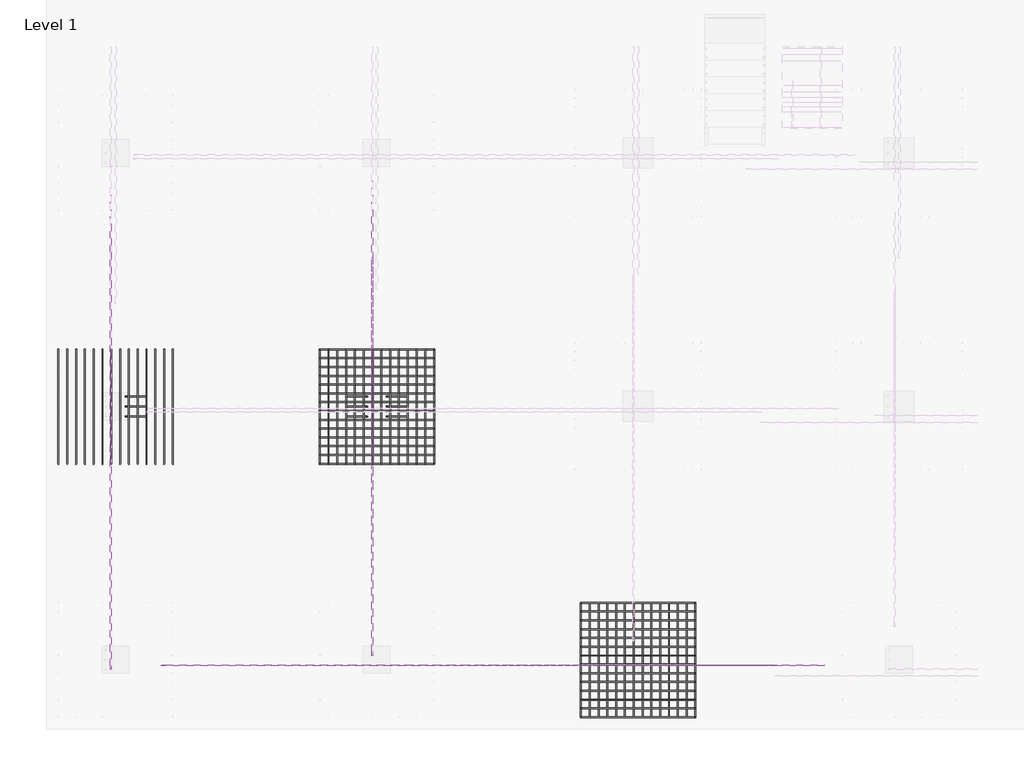
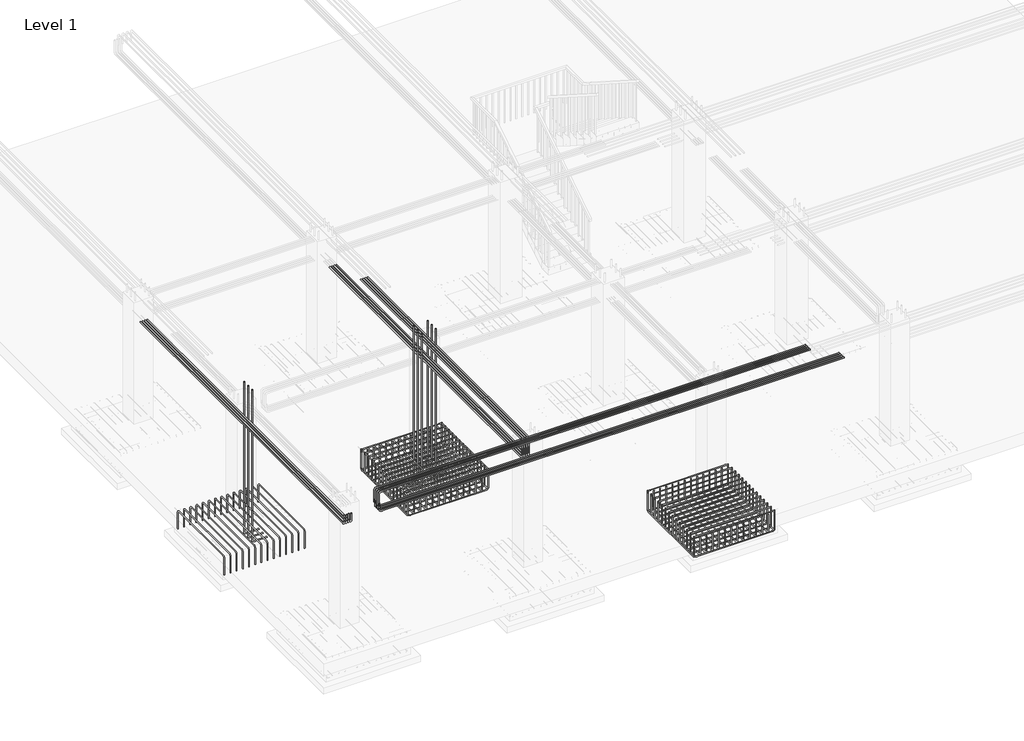
# One storey, part 4 of 17: 21 reinforcing bars.
"""IFC4 building model written with IfcOpenShell, lengths in millimetres."""

from ifc_helpers import new_model, si_unit, point, frame, origin, place, context, project, spatial, polyline, circle_curve, trimmed, segment, composite_curve, source, transform, mapped, element, save
from ifc_brep_helpers import swept_disk

model = new_model("IFC4")

# Units and contexts
model_context = context("Model", 3, world=origin())
ifc_project = project(units=[si_unit("LENGTHUNIT", "METRE", prefix="MILLI")], contexts=[model_context])

# Site, building, storey
site = spatial("IfcSite", under=ifc_project)
building = spatial("IfcBuilding", under=site)
storey = spatial("IfcBuildingStorey", under=building, Name="Level 1", Elevation=0.0)

# Reinforcing bars
placement = place(None, origin())
reinforcing_bar_shape = source(origin(), model_context, "Body", "SolidModel", [
    swept_disk(composite_curve([segment(polyline([(-13686.3632003, 636.009457, -504.0), (-13686.3632003, 636.009457, -96.0)]), True, "CONTINUOUS"), segment(trimmed(circle_curve(frame((-13686.3632003, 588.009457, -96.0), z_axis=(1.0, 0.0, 0.0), x_axis=(0.0, 48.0, 0.0)), 48.0), [point((-13686.3632003, 636.009457, -96.0))], [point((-13686.3632003, 588.009457, -48.0))], True, "CARTESIAN"), True, "CONTINUOUS"), segment(polyline([(-13686.3632003, 588.009457, -48.0), (-13686.3632003, -1219.990543, -48.0)]), True, "CONTINUOUS"), segment(trimmed(circle_curve(frame((-13686.3632003, -1219.990543, -96.0), z_axis=(1.0, 0.0, 0.0), x_axis=(0.0, 0.0, 48.0)), 48.0), [point((-13686.3632003, -1219.990543, -48.0))], [point((-13686.3632003, -1267.990543, -96.0))], True, "CARTESIAN"), True, "CONTINUOUS"), segment(polyline([(-13686.3632003, -1267.990543, -96.0), (-13686.3632003, -1267.990543, -504.0)]), True, "CONTINUOUS")], self_intersect=False), 8.0),
])
element("IfcReinforcingBar", 1, at=placement, inside=storey, context=model_context, shape_type="MappedRepresentation", body=[
    mapped(reinforcing_bar_shape, transform((0.0, 0.0, 0.0), x_axis=(1.0, 0.0, 0.0), y_axis=(0.0, 1.0, 0.0), z_axis=(0.0, 0.0, 1.0))),
    mapped(reinforcing_bar_shape, transform((146.4615385, 0.0, 0.0), x_axis=(1.0, 0.0, 0.0), y_axis=(0.0, 1.0, 0.0), z_axis=(0.0, 0.0, 1.0))),
    mapped(reinforcing_bar_shape, transform((292.9230769, 0.0, 0.0), x_axis=(1.0, 0.0, 0.0), y_axis=(0.0, 1.0, 0.0), z_axis=(0.0, 0.0, 1.0))),
    mapped(reinforcing_bar_shape, transform((439.3846154, 0.0, 0.0), x_axis=(1.0, 0.0, 0.0), y_axis=(0.0, 1.0, 0.0), z_axis=(0.0, 0.0, 1.0))),
    mapped(reinforcing_bar_shape, transform((585.8461538, 0.0, 0.0), x_axis=(1.0, 0.0, 0.0), y_axis=(0.0, 1.0, 0.0), z_axis=(0.0, 0.0, 1.0))),
    mapped(reinforcing_bar_shape, transform((732.3076923, 0.0, 0.0), x_axis=(1.0, 0.0, 0.0), y_axis=(0.0, 1.0, 0.0), z_axis=(0.0, 0.0, 1.0))),
    mapped(reinforcing_bar_shape, transform((878.7692308, 0.0, 0.0), x_axis=(1.0, 0.0, 0.0), y_axis=(0.0, 1.0, 0.0), z_axis=(0.0, 0.0, 1.0))),
    mapped(reinforcing_bar_shape, transform((1025.2307692, 0.0, 0.0), x_axis=(1.0, 0.0, 0.0), y_axis=(0.0, 1.0, 0.0), z_axis=(0.0, 0.0, 1.0))),
    mapped(reinforcing_bar_shape, transform((1171.6923077, 0.0, 0.0), x_axis=(1.0, 0.0, 0.0), y_axis=(0.0, 1.0, 0.0), z_axis=(0.0, 0.0, 1.0))),
    mapped(reinforcing_bar_shape, transform((1318.1538462, 0.0, 0.0), x_axis=(1.0, 0.0, 0.0), y_axis=(0.0, 1.0, 0.0), z_axis=(0.0, 0.0, 1.0))),
    mapped(reinforcing_bar_shape, transform((1464.6153846, 0.0, 0.0), x_axis=(1.0, 0.0, 0.0), y_axis=(0.0, 1.0, 0.0), z_axis=(0.0, 0.0, 1.0))),
    mapped(reinforcing_bar_shape, transform((1611.0769231, 0.0, 0.0), x_axis=(1.0, 0.0, 0.0), y_axis=(0.0, 1.0, 0.0), z_axis=(0.0, 0.0, 1.0))),
    mapped(reinforcing_bar_shape, transform((1757.5384615, 0.0, 0.0), x_axis=(1.0, 0.0, 0.0), y_axis=(0.0, 1.0, 0.0), z_axis=(0.0, 0.0, 1.0))),
    mapped(reinforcing_bar_shape, transform((1904.0, 0.0, 0.0), x_axis=(1.0, 0.0, 0.0), y_axis=(0.0, 1.0, 0.0), z_axis=(0.0, 0.0, 1.0))),
])
reinforcing_bar_2_shape = source(origin(), model_context, "Body", "SolidModel", [
    swept_disk(composite_curve([segment(polyline([(-12221.7478157, -481.490543, -550.0), (-12518.8632003, -481.490543, -550.0)]), True, "CONTINUOUS"), segment(trimmed(circle_curve(frame((-12518.8632003, -481.490543, -500.0), z_axis=(0.0, 1.0, 0.0), x_axis=(0.0, 0.0, -50.0)), 50.0), [point((-12518.8632003, -481.490543, -550.0))], [point((-12568.8632003, -481.490543, -500.0))], True, "CARTESIAN"), True, "CONTINUOUS"), segment(polyline([(-12568.8632003, -481.490543, -500.0), (-12568.8632003, -481.490543, 3260.0)]), True, "CONTINUOUS")], self_intersect=False), 10.0),
])
element("IfcReinforcingBar", 2, at=placement, inside=storey, context=model_context, shape_type="MappedRepresentation", body=[
    mapped(reinforcing_bar_2_shape, transform((0.0, 0.0, 0.0), x_axis=(1.0, 0.0, 0.0), y_axis=(0.0, 1.0, 0.0), z_axis=(0.0, 0.0, 1.0))),
    mapped(reinforcing_bar_2_shape, transform((0.0, 165.5, 0.0), x_axis=(1.0, 0.0, 0.0), y_axis=(0.0, 1.0, 0.0), z_axis=(0.0, 0.0, 1.0))),
    mapped(reinforcing_bar_2_shape, transform((0.0, 331.0, 0.0), x_axis=(1.0, 0.0, 0.0), y_axis=(0.0, 1.0, 0.0), z_axis=(0.0, 0.0, 1.0))),
])
reinforcing_bar_3_shape = source(origin(), model_context, "Body", "SolidModel", [
    swept_disk(composite_curve([segment(polyline([(-9341.3632003, 636.009457, -40.0), (-9341.3632003, 636.009457, -504.0)]), True, "CONTINUOUS"), segment(trimmed(circle_curve(frame((-9293.3632003, 636.009457, -504.0), z_axis=(0.0, -1.0, 0.0), x_axis=(-48.0, 0.0, 0.0)), 48.0), [point((-9341.3632003, 636.009457, -504.0))], [point((-9293.3632003, 636.009457, -552.0))], True, "CARTESIAN"), True, "CONTINUOUS"), segment(polyline([(-9293.3632003, 636.009457, -552.0), (-7485.3632003, 636.009457, -552.0)]), True, "CONTINUOUS"), segment(trimmed(circle_curve(frame((-7485.3632003, 636.009457, -504.0), z_axis=(0.0, -1.0, 0.0), x_axis=(0.0, 0.0, -48.0)), 48.0), [point((-7485.3632003, 636.009457, -552.0))], [point((-7437.3632003, 636.009457, -504.0))], True, "CARTESIAN"), True, "CONTINUOUS"), segment(polyline([(-7437.3632003, 636.009457, -504.0), (-7437.3632003, 636.009457, -40.0)]), True, "CONTINUOUS")], self_intersect=False), 8.0),
])
element("IfcReinforcingBar", 3, at=placement, inside=storey, context=model_context, shape_type="MappedRepresentation", body=[
    mapped(reinforcing_bar_3_shape, transform((0.0, 0.0, 0.0), x_axis=(1.0, 0.0, 0.0), y_axis=(0.0, 1.0, 0.0), z_axis=(0.0, 0.0, 1.0))),
    mapped(reinforcing_bar_3_shape, transform((0.0, -146.4615385, 0.0), x_axis=(1.0, 0.0, 0.0), y_axis=(0.0, 1.0, 0.0), z_axis=(0.0, 0.0, 1.0))),
    mapped(reinforcing_bar_3_shape, transform((0.0, -292.9230769, 0.0), x_axis=(1.0, 0.0, 0.0), y_axis=(0.0, 1.0, 0.0), z_axis=(0.0, 0.0, 1.0))),
    mapped(reinforcing_bar_3_shape, transform((0.0, -439.3846154, 0.0), x_axis=(1.0, 0.0, 0.0), y_axis=(0.0, 1.0, 0.0), z_axis=(0.0, 0.0, 1.0))),
    mapped(reinforcing_bar_3_shape, transform((0.0, -585.8461538, 0.0), x_axis=(1.0, 0.0, 0.0), y_axis=(0.0, 1.0, 0.0), z_axis=(0.0, 0.0, 1.0))),
    mapped(reinforcing_bar_3_shape, transform((0.0, -732.3076923, 0.0), x_axis=(1.0, 0.0, 0.0), y_axis=(0.0, 1.0, 0.0), z_axis=(0.0, 0.0, 1.0))),
    mapped(reinforcing_bar_3_shape, transform((0.0, -878.7692308, 0.0), x_axis=(1.0, 0.0, 0.0), y_axis=(0.0, 1.0, 0.0), z_axis=(0.0, 0.0, 1.0))),
    mapped(reinforcing_bar_3_shape, transform((0.0, -1025.2307692, 0.0), x_axis=(1.0, 0.0, 0.0), y_axis=(0.0, 1.0, 0.0), z_axis=(0.0, 0.0, 1.0))),
    mapped(reinforcing_bar_3_shape, transform((0.0, -1171.6923077, 0.0), x_axis=(1.0, 0.0, 0.0), y_axis=(0.0, 1.0, 0.0), z_axis=(0.0, 0.0, 1.0))),
    mapped(reinforcing_bar_3_shape, transform((0.0, -1318.1538462, 0.0), x_axis=(1.0, 0.0, 0.0), y_axis=(0.0, 1.0, 0.0), z_axis=(0.0, 0.0, 1.0))),
    mapped(reinforcing_bar_3_shape, transform((0.0, -1464.6153846, 0.0), x_axis=(1.0, 0.0, 0.0), y_axis=(0.0, 1.0, 0.0), z_axis=(0.0, 0.0, 1.0))),
    mapped(reinforcing_bar_3_shape, transform((0.0, -1611.0769231, 0.0), x_axis=(1.0, 0.0, 0.0), y_axis=(0.0, 1.0, 0.0), z_axis=(0.0, 0.0, 1.0))),
    mapped(reinforcing_bar_3_shape, transform((0.0, -1757.5384615, 0.0), x_axis=(1.0, 0.0, 0.0), y_axis=(0.0, 1.0, 0.0), z_axis=(0.0, 0.0, 1.0))),
    mapped(reinforcing_bar_3_shape, transform((0.0, -1904.0, 0.0), x_axis=(1.0, 0.0, 0.0), y_axis=(0.0, 1.0, 0.0), z_axis=(0.0, 0.0, 1.0))),
])
reinforcing_bar_4_shape = source(origin(), model_context, "Body", "SolidModel", [
    swept_disk(composite_curve([segment(polyline([(-9341.3632003, -1267.990543, -504.0), (-9341.3632003, -1267.990543, -96.0)]), True, "CONTINUOUS"), segment(trimmed(circle_curve(frame((-9293.3632003, -1267.990543, -96.0), z_axis=(0.0, 1.0, 0.0), x_axis=(-48.0, 0.0, 0.0)), 48.0), [point((-9341.3632003, -1267.990543, -96.0))], [point((-9293.3632003, -1267.990543, -48.0))], True, "CARTESIAN"), True, "CONTINUOUS"), segment(polyline([(-9293.3632003, -1267.990543, -48.0), (-7485.3632003, -1267.990543, -48.0)]), True, "CONTINUOUS"), segment(trimmed(circle_curve(frame((-7485.3632003, -1267.990543, -96.0), z_axis=(0.0, 1.0, 0.0), x_axis=(0.0, 0.0, 48.0)), 48.0), [point((-7485.3632003, -1267.990543, -48.0))], [point((-7437.3632003, -1267.990543, -96.0))], True, "CARTESIAN"), True, "CONTINUOUS"), segment(polyline([(-7437.3632003, -1267.990543, -96.0), (-7437.3632003, -1267.990543, -504.0)]), True, "CONTINUOUS")], self_intersect=False), 8.0),
])
element("IfcReinforcingBar", 4, at=placement, inside=storey, context=model_context, shape_type="MappedRepresentation", body=[
    mapped(reinforcing_bar_4_shape, transform((0.0, 0.0, 0.0), x_axis=(1.0, 0.0, 0.0), y_axis=(0.0, 1.0, 0.0), z_axis=(0.0, 0.0, 1.0))),
    mapped(reinforcing_bar_4_shape, transform((0.0, 146.4615385, 0.0), x_axis=(1.0, 0.0, 0.0), y_axis=(0.0, 1.0, 0.0), z_axis=(0.0, 0.0, 1.0))),
    mapped(reinforcing_bar_4_shape, transform((0.0, 292.9230769, 0.0), x_axis=(1.0, 0.0, 0.0), y_axis=(0.0, 1.0, 0.0), z_axis=(0.0, 0.0, 1.0))),
    mapped(reinforcing_bar_4_shape, transform((0.0, 439.3846154, 0.0), x_axis=(1.0, 0.0, 0.0), y_axis=(0.0, 1.0, 0.0), z_axis=(0.0, 0.0, 1.0))),
    mapped(reinforcing_bar_4_shape, transform((0.0, 585.8461538, 0.0), x_axis=(1.0, 0.0, 0.0), y_axis=(0.0, 1.0, 0.0), z_axis=(0.0, 0.0, 1.0))),
    mapped(reinforcing_bar_4_shape, transform((0.0, 732.3076923, 0.0), x_axis=(1.0, 0.0, 0.0), y_axis=(0.0, 1.0, 0.0), z_axis=(0.0, 0.0, 1.0))),
    mapped(reinforcing_bar_4_shape, transform((0.0, 878.7692308, 0.0), x_axis=(1.0, 0.0, 0.0), y_axis=(0.0, 1.0, 0.0), z_axis=(0.0, 0.0, 1.0))),
    mapped(reinforcing_bar_4_shape, transform((0.0, 1025.2307692, 0.0), x_axis=(1.0, 0.0, 0.0), y_axis=(0.0, 1.0, 0.0), z_axis=(0.0, 0.0, 1.0))),
    mapped(reinforcing_bar_4_shape, transform((0.0, 1171.6923077, 0.0), x_axis=(1.0, 0.0, 0.0), y_axis=(0.0, 1.0, 0.0), z_axis=(0.0, 0.0, 1.0))),
    mapped(reinforcing_bar_4_shape, transform((0.0, 1318.1538462, 0.0), x_axis=(1.0, 0.0, 0.0), y_axis=(0.0, 1.0, 0.0), z_axis=(0.0, 0.0, 1.0))),
    mapped(reinforcing_bar_4_shape, transform((0.0, 1464.6153846, 0.0), x_axis=(1.0, 0.0, 0.0), y_axis=(0.0, 1.0, 0.0), z_axis=(0.0, 0.0, 1.0))),
    mapped(reinforcing_bar_4_shape, transform((0.0, 1611.0769231, 0.0), x_axis=(1.0, 0.0, 0.0), y_axis=(0.0, 1.0, 0.0), z_axis=(0.0, 0.0, 1.0))),
    mapped(reinforcing_bar_4_shape, transform((0.0, 1757.5384615, 0.0), x_axis=(1.0, 0.0, 0.0), y_axis=(0.0, 1.0, 0.0), z_axis=(0.0, 0.0, 1.0))),
    mapped(reinforcing_bar_4_shape, transform((0.0, 1904.0, 0.0), x_axis=(1.0, 0.0, 0.0), y_axis=(0.0, 1.0, 0.0), z_axis=(0.0, 0.0, 1.0))),
])
reinforcing_bar_5_shape = source(origin(), model_context, "Body", "SolidModel", [
    swept_disk(composite_curve([segment(polyline([(-7437.3632003, 636.009457, -96.0), (-7437.3632003, 636.009457, -504.0)]), True, "CONTINUOUS"), segment(trimmed(circle_curve(frame((-7437.3632003, 588.009457, -504.0), z_axis=(-1.0, 0.0, 0.0), x_axis=(0.0, 48.0, 0.0)), 48.0), [point((-7437.3632003, 636.009457, -504.0))], [point((-7437.3632003, 588.009457, -552.0))], True, "CARTESIAN"), True, "CONTINUOUS"), segment(polyline([(-7437.3632003, 588.009457, -552.0), (-7437.3632003, -1219.990543, -552.0)]), True, "CONTINUOUS"), segment(trimmed(circle_curve(frame((-7437.3632003, -1219.990543, -504.0), z_axis=(-1.0, 0.0, 0.0), x_axis=(0.0, 0.0, -48.0)), 48.0), [point((-7437.3632003, -1219.990543, -552.0))], [point((-7437.3632003, -1267.990543, -504.0))], True, "CARTESIAN"), True, "CONTINUOUS"), segment(polyline([(-7437.3632003, -1267.990543, -504.0), (-7437.3632003, -1267.990543, -96.0)]), True, "CONTINUOUS")], self_intersect=False), 8.0),
])
element("IfcReinforcingBar", 5, at=placement, inside=storey, context=model_context, shape_type="MappedRepresentation", body=[
    mapped(reinforcing_bar_5_shape, transform((0.0, 0.0, 0.0), x_axis=(1.0, 0.0, 0.0), y_axis=(0.0, 1.0, 0.0), z_axis=(0.0, 0.0, 1.0))),
    mapped(reinforcing_bar_5_shape, transform((-146.4615385, 0.0, 0.0), x_axis=(1.0, 0.0, 0.0), y_axis=(0.0, 1.0, 0.0), z_axis=(0.0, 0.0, 1.0))),
    mapped(reinforcing_bar_5_shape, transform((-292.9230769, 0.0, 0.0), x_axis=(1.0, 0.0, 0.0), y_axis=(0.0, 1.0, 0.0), z_axis=(0.0, 0.0, 1.0))),
    mapped(reinforcing_bar_5_shape, transform((-439.3846154, 0.0, 0.0), x_axis=(1.0, 0.0, 0.0), y_axis=(0.0, 1.0, 0.0), z_axis=(0.0, 0.0, 1.0))),
    mapped(reinforcing_bar_5_shape, transform((-585.8461538, 0.0, 0.0), x_axis=(1.0, 0.0, 0.0), y_axis=(0.0, 1.0, 0.0), z_axis=(0.0, 0.0, 1.0))),
    mapped(reinforcing_bar_5_shape, transform((-732.3076923, 0.0, 0.0), x_axis=(1.0, 0.0, 0.0), y_axis=(0.0, 1.0, 0.0), z_axis=(0.0, 0.0, 1.0))),
    mapped(reinforcing_bar_5_shape, transform((-878.7692308, 0.0, 0.0), x_axis=(1.0, 0.0, 0.0), y_axis=(0.0, 1.0, 0.0), z_axis=(0.0, 0.0, 1.0))),
    mapped(reinforcing_bar_5_shape, transform((-1025.2307692, 0.0, 0.0), x_axis=(1.0, 0.0, 0.0), y_axis=(0.0, 1.0, 0.0), z_axis=(0.0, 0.0, 1.0))),
    mapped(reinforcing_bar_5_shape, transform((-1171.6923077, 0.0, 0.0), x_axis=(1.0, 0.0, 0.0), y_axis=(0.0, 1.0, 0.0), z_axis=(0.0, 0.0, 1.0))),
    mapped(reinforcing_bar_5_shape, transform((-1318.1538462, 0.0, 0.0), x_axis=(1.0, 0.0, 0.0), y_axis=(0.0, 1.0, 0.0), z_axis=(0.0, 0.0, 1.0))),
    mapped(reinforcing_bar_5_shape, transform((-1464.6153846, 0.0, 0.0), x_axis=(1.0, 0.0, 0.0), y_axis=(0.0, 1.0, 0.0), z_axis=(0.0, 0.0, 1.0))),
    mapped(reinforcing_bar_5_shape, transform((-1611.0769231, 0.0, 0.0), x_axis=(1.0, 0.0, 0.0), y_axis=(0.0, 1.0, 0.0), z_axis=(0.0, 0.0, 1.0))),
    mapped(reinforcing_bar_5_shape, transform((-1757.5384615, 0.0, 0.0), x_axis=(1.0, 0.0, 0.0), y_axis=(0.0, 1.0, 0.0), z_axis=(0.0, 0.0, 1.0))),
    mapped(reinforcing_bar_5_shape, transform((-1904.0, 0.0, 0.0), x_axis=(1.0, 0.0, 0.0), y_axis=(0.0, 1.0, 0.0), z_axis=(0.0, 0.0, 1.0))),
])
reinforcing_bar_6_shape = source(origin(), model_context, "Body", "SolidModel", [
    swept_disk(composite_curve([segment(polyline([(-9341.3632003, 636.009457, -504.0), (-9341.3632003, 636.009457, -96.0)]), True, "CONTINUOUS"), segment(trimmed(circle_curve(frame((-9341.3632003, 588.009457, -96.0), z_axis=(1.0, 0.0, 0.0), x_axis=(0.0, 48.0, 0.0)), 48.0), [point((-9341.3632003, 636.009457, -96.0))], [point((-9341.3632003, 588.009457, -48.0))], True, "CARTESIAN"), True, "CONTINUOUS"), segment(polyline([(-9341.3632003, 588.009457, -48.0), (-9341.3632003, -1219.990543, -48.0)]), True, "CONTINUOUS"), segment(trimmed(circle_curve(frame((-9341.3632003, -1219.990543, -96.0), z_axis=(1.0, 0.0, 0.0), x_axis=(0.0, 0.0, 48.0)), 48.0), [point((-9341.3632003, -1219.990543, -48.0))], [point((-9341.3632003, -1267.990543, -96.0))], True, "CARTESIAN"), True, "CONTINUOUS"), segment(polyline([(-9341.3632003, -1267.990543, -96.0), (-9341.3632003, -1267.990543, -504.0)]), True, "CONTINUOUS")], self_intersect=False), 8.0),
])
element("IfcReinforcingBar", 6, at=placement, inside=storey, context=model_context, shape_type="MappedRepresentation", body=[
    mapped(reinforcing_bar_6_shape, transform((0.0, 0.0, 0.0), x_axis=(1.0, 0.0, 0.0), y_axis=(0.0, 1.0, 0.0), z_axis=(0.0, 0.0, 1.0))),
    mapped(reinforcing_bar_6_shape, transform((146.4615385, 0.0, 0.0), x_axis=(1.0, 0.0, 0.0), y_axis=(0.0, 1.0, 0.0), z_axis=(0.0, 0.0, 1.0))),
    mapped(reinforcing_bar_6_shape, transform((292.9230769, 0.0, 0.0), x_axis=(1.0, 0.0, 0.0), y_axis=(0.0, 1.0, 0.0), z_axis=(0.0, 0.0, 1.0))),
    mapped(reinforcing_bar_6_shape, transform((439.3846154, 0.0, 0.0), x_axis=(1.0, 0.0, 0.0), y_axis=(0.0, 1.0, 0.0), z_axis=(0.0, 0.0, 1.0))),
    mapped(reinforcing_bar_6_shape, transform((585.8461538, 0.0, 0.0), x_axis=(1.0, 0.0, 0.0), y_axis=(0.0, 1.0, 0.0), z_axis=(0.0, 0.0, 1.0))),
    mapped(reinforcing_bar_6_shape, transform((732.3076923, 0.0, 0.0), x_axis=(1.0, 0.0, 0.0), y_axis=(0.0, 1.0, 0.0), z_axis=(0.0, 0.0, 1.0))),
    mapped(reinforcing_bar_6_shape, transform((878.7692308, 0.0, 0.0), x_axis=(1.0, 0.0, 0.0), y_axis=(0.0, 1.0, 0.0), z_axis=(0.0, 0.0, 1.0))),
    mapped(reinforcing_bar_6_shape, transform((1025.2307692, 0.0, 0.0), x_axis=(1.0, 0.0, 0.0), y_axis=(0.0, 1.0, 0.0), z_axis=(0.0, 0.0, 1.0))),
    mapped(reinforcing_bar_6_shape, transform((1171.6923077, 0.0, 0.0), x_axis=(1.0, 0.0, 0.0), y_axis=(0.0, 1.0, 0.0), z_axis=(0.0, 0.0, 1.0))),
    mapped(reinforcing_bar_6_shape, transform((1318.1538462, 0.0, 0.0), x_axis=(1.0, 0.0, 0.0), y_axis=(0.0, 1.0, 0.0), z_axis=(0.0, 0.0, 1.0))),
    mapped(reinforcing_bar_6_shape, transform((1464.6153846, 0.0, 0.0), x_axis=(1.0, 0.0, 0.0), y_axis=(0.0, 1.0, 0.0), z_axis=(0.0, 0.0, 1.0))),
    mapped(reinforcing_bar_6_shape, transform((1611.0769231, 0.0, 0.0), x_axis=(1.0, 0.0, 0.0), y_axis=(0.0, 1.0, 0.0), z_axis=(0.0, 0.0, 1.0))),
    mapped(reinforcing_bar_6_shape, transform((1757.5384615, 0.0, 0.0), x_axis=(1.0, 0.0, 0.0), y_axis=(0.0, 1.0, 0.0), z_axis=(0.0, 0.0, 1.0))),
    mapped(reinforcing_bar_6_shape, transform((1904.0, 0.0, 0.0), x_axis=(1.0, 0.0, 0.0), y_axis=(0.0, 1.0, 0.0), z_axis=(0.0, 0.0, 1.0))),
])
reinforcing_bar_7_shape = source(origin(), model_context, "Body", "SolidModel", [
    swept_disk(composite_curve([segment(polyline([(-8901.9785849, -150.490543, -550.0), (-8604.8632003, -150.490543, -550.0)]), True, "CONTINUOUS"), segment(trimmed(circle_curve(frame((-8604.8632003, -150.490543, -500.0), z_axis=(0.0, -1.0, 0.0), x_axis=(0.0, 0.0, -50.0)), 50.0), [point((-8604.8632003, -150.490543, -550.0))], [point((-8554.8632003, -150.490543, -500.0))], True, "CARTESIAN"), True, "CONTINUOUS"), segment(polyline([(-8554.8632003, -150.490543, -500.0), (-8554.8632003, -150.490543, 3260.0)]), True, "CONTINUOUS")], self_intersect=False), 10.0),
])
element("IfcReinforcingBar", 7, at=placement, inside=storey, context=model_context, shape_type="MappedRepresentation", body=[
    mapped(reinforcing_bar_7_shape, transform((0.0, 0.0, 0.0), x_axis=(1.0, 0.0, 0.0), y_axis=(0.0, 1.0, 0.0), z_axis=(0.0, 0.0, 1.0))),
    mapped(reinforcing_bar_7_shape, transform((0.0, -165.5, 0.0), x_axis=(1.0, 0.0, 0.0), y_axis=(0.0, 1.0, 0.0), z_axis=(0.0, 0.0, 1.0))),
    mapped(reinforcing_bar_7_shape, transform((0.0, -331.0, 0.0), x_axis=(1.0, 0.0, 0.0), y_axis=(0.0, 1.0, 0.0), z_axis=(0.0, 0.0, 1.0))),
])
reinforcing_bar_8_shape = source(origin(), model_context, "Body", "SolidModel", [
    swept_disk(composite_curve([segment(polyline([(-7876.7478157, -481.490543, -550.0), (-8173.8632003, -481.490543, -550.0)]), True, "CONTINUOUS"), segment(trimmed(circle_curve(frame((-8173.8632003, -481.490543, -500.0), z_axis=(0.0, 1.0, 0.0), x_axis=(0.0, 0.0, -50.0)), 50.0), [point((-8173.8632003, -481.490543, -550.0))], [point((-8223.8632003, -481.490543, -500.0))], True, "CARTESIAN"), True, "CONTINUOUS"), segment(polyline([(-8223.8632003, -481.490543, -500.0), (-8223.8632003, -481.490543, 3260.0)]), True, "CONTINUOUS")], self_intersect=False), 10.0),
])
element("IfcReinforcingBar", 8, at=placement, inside=storey, context=model_context, shape_type="MappedRepresentation", body=[
    mapped(reinforcing_bar_8_shape, transform((0.0, 0.0, 0.0), x_axis=(1.0, 0.0, 0.0), y_axis=(0.0, 1.0, 0.0), z_axis=(0.0, 0.0, 1.0))),
    mapped(reinforcing_bar_8_shape, transform((0.0, 165.5, 0.0), x_axis=(1.0, 0.0, 0.0), y_axis=(0.0, 1.0, 0.0), z_axis=(0.0, 0.0, 1.0))),
    mapped(reinforcing_bar_8_shape, transform((0.0, 331.0, 0.0), x_axis=(1.0, 0.0, 0.0), y_axis=(0.0, 1.0, 0.0), z_axis=(0.0, 0.0, 1.0))),
])
reinforcing_bar_9_shape = source(origin(), model_context, "Body", "SolidModel", [
    swept_disk(composite_curve([segment(polyline([(-4996.3632003, -3580.990543, -40.0), (-4996.3632003, -3580.990543, -504.0)]), True, "CONTINUOUS"), segment(trimmed(circle_curve(frame((-4948.3632003, -3580.990543, -504.0), z_axis=(0.0, -1.0, 0.0), x_axis=(-48.0, 0.0, 0.0)), 48.0), [point((-4996.3632003, -3580.990543, -504.0))], [point((-4948.3632003, -3580.990543, -552.0))], True, "CARTESIAN"), True, "CONTINUOUS"), segment(polyline([(-4948.3632003, -3580.990543, -552.0), (-3140.3632003, -3580.990543, -552.0)]), True, "CONTINUOUS"), segment(trimmed(circle_curve(frame((-3140.3632003, -3580.990543, -504.0), z_axis=(0.0, -1.0, 0.0), x_axis=(0.0, 0.0, -48.0)), 48.0), [point((-3140.3632003, -3580.990543, -552.0))], [point((-3092.3632003, -3580.990543, -504.0))], True, "CARTESIAN"), True, "CONTINUOUS"), segment(polyline([(-3092.3632003, -3580.990543, -504.0), (-3092.3632003, -3580.990543, -40.0)]), True, "CONTINUOUS")], self_intersect=False), 8.0),
])
element("IfcReinforcingBar", 9, at=placement, inside=storey, context=model_context, shape_type="MappedRepresentation", body=[
    mapped(reinforcing_bar_9_shape, transform((0.0, 0.0, 0.0), x_axis=(1.0, 0.0, 0.0), y_axis=(0.0, 1.0, 0.0), z_axis=(0.0, 0.0, 1.0))),
    mapped(reinforcing_bar_9_shape, transform((0.0, -146.4615385, 0.0), x_axis=(1.0, 0.0, 0.0), y_axis=(0.0, 1.0, 0.0), z_axis=(0.0, 0.0, 1.0))),
    mapped(reinforcing_bar_9_shape, transform((0.0, -292.9230769, 0.0), x_axis=(1.0, 0.0, 0.0), y_axis=(0.0, 1.0, 0.0), z_axis=(0.0, 0.0, 1.0))),
    mapped(reinforcing_bar_9_shape, transform((0.0, -439.3846154, 0.0), x_axis=(1.0, 0.0, 0.0), y_axis=(0.0, 1.0, 0.0), z_axis=(0.0, 0.0, 1.0))),
    mapped(reinforcing_bar_9_shape, transform((0.0, -585.8461538, 0.0), x_axis=(1.0, 0.0, 0.0), y_axis=(0.0, 1.0, 0.0), z_axis=(0.0, 0.0, 1.0))),
    mapped(reinforcing_bar_9_shape, transform((0.0, -732.3076923, 0.0), x_axis=(1.0, 0.0, 0.0), y_axis=(0.0, 1.0, 0.0), z_axis=(0.0, 0.0, 1.0))),
    mapped(reinforcing_bar_9_shape, transform((0.0, -878.7692308, 0.0), x_axis=(1.0, 0.0, 0.0), y_axis=(0.0, 1.0, 0.0), z_axis=(0.0, 0.0, 1.0))),
    mapped(reinforcing_bar_9_shape, transform((0.0, -1025.2307692, 0.0), x_axis=(1.0, 0.0, 0.0), y_axis=(0.0, 1.0, 0.0), z_axis=(0.0, 0.0, 1.0))),
    mapped(reinforcing_bar_9_shape, transform((0.0, -1171.6923077, 0.0), x_axis=(1.0, 0.0, 0.0), y_axis=(0.0, 1.0, 0.0), z_axis=(0.0, 0.0, 1.0))),
    mapped(reinforcing_bar_9_shape, transform((0.0, -1318.1538462, 0.0), x_axis=(1.0, 0.0, 0.0), y_axis=(0.0, 1.0, 0.0), z_axis=(0.0, 0.0, 1.0))),
    mapped(reinforcing_bar_9_shape, transform((0.0, -1464.6153846, 0.0), x_axis=(1.0, 0.0, 0.0), y_axis=(0.0, 1.0, 0.0), z_axis=(0.0, 0.0, 1.0))),
    mapped(reinforcing_bar_9_shape, transform((0.0, -1611.0769231, 0.0), x_axis=(1.0, 0.0, 0.0), y_axis=(0.0, 1.0, 0.0), z_axis=(0.0, 0.0, 1.0))),
    mapped(reinforcing_bar_9_shape, transform((0.0, -1757.5384615, 0.0), x_axis=(1.0, 0.0, 0.0), y_axis=(0.0, 1.0, 0.0), z_axis=(0.0, 0.0, 1.0))),
    mapped(reinforcing_bar_9_shape, transform((0.0, -1904.0, 0.0), x_axis=(1.0, 0.0, 0.0), y_axis=(0.0, 1.0, 0.0), z_axis=(0.0, 0.0, 1.0))),
])
reinforcing_bar_10_shape = source(origin(), model_context, "Body", "SolidModel", [
    swept_disk(composite_curve([segment(polyline([(-4996.3632003, -5484.990543, -504.0), (-4996.3632003, -5484.990543, -96.0)]), True, "CONTINUOUS"), segment(trimmed(circle_curve(frame((-4948.3632003, -5484.990543, -96.0), z_axis=(0.0, 1.0, 0.0), x_axis=(-48.0, 0.0, 0.0)), 48.0), [point((-4996.3632003, -5484.990543, -96.0))], [point((-4948.3632003, -5484.990543, -48.0))], True, "CARTESIAN"), True, "CONTINUOUS"), segment(polyline([(-4948.3632003, -5484.990543, -48.0), (-3140.3632003, -5484.990543, -48.0)]), True, "CONTINUOUS"), segment(trimmed(circle_curve(frame((-3140.3632003, -5484.990543, -96.0), z_axis=(0.0, 1.0, 0.0), x_axis=(0.0, 0.0, 48.0)), 48.0), [point((-3140.3632003, -5484.990543, -48.0))], [point((-3092.3632003, -5484.990543, -96.0))], True, "CARTESIAN"), True, "CONTINUOUS"), segment(polyline([(-3092.3632003, -5484.990543, -96.0), (-3092.3632003, -5484.990543, -504.0)]), True, "CONTINUOUS")], self_intersect=False), 8.0),
])
element("IfcReinforcingBar", 10, at=placement, inside=storey, context=model_context, shape_type="MappedRepresentation", body=[
    mapped(reinforcing_bar_10_shape, transform((0.0, 0.0, 0.0), x_axis=(1.0, 0.0, 0.0), y_axis=(0.0, 1.0, 0.0), z_axis=(0.0, 0.0, 1.0))),
    mapped(reinforcing_bar_10_shape, transform((0.0, 146.4615385, 0.0), x_axis=(1.0, 0.0, 0.0), y_axis=(0.0, 1.0, 0.0), z_axis=(0.0, 0.0, 1.0))),
    mapped(reinforcing_bar_10_shape, transform((0.0, 292.9230769, 0.0), x_axis=(1.0, 0.0, 0.0), y_axis=(0.0, 1.0, 0.0), z_axis=(0.0, 0.0, 1.0))),
    mapped(reinforcing_bar_10_shape, transform((0.0, 439.3846154, 0.0), x_axis=(1.0, 0.0, 0.0), y_axis=(0.0, 1.0, 0.0), z_axis=(0.0, 0.0, 1.0))),
    mapped(reinforcing_bar_10_shape, transform((0.0, 585.8461538, 0.0), x_axis=(1.0, 0.0, 0.0), y_axis=(0.0, 1.0, 0.0), z_axis=(0.0, 0.0, 1.0))),
    mapped(reinforcing_bar_10_shape, transform((0.0, 732.3076923, 0.0), x_axis=(1.0, 0.0, 0.0), y_axis=(0.0, 1.0, 0.0), z_axis=(0.0, 0.0, 1.0))),
    mapped(reinforcing_bar_10_shape, transform((0.0, 878.7692308, 0.0), x_axis=(1.0, 0.0, 0.0), y_axis=(0.0, 1.0, 0.0), z_axis=(0.0, 0.0, 1.0))),
    mapped(reinforcing_bar_10_shape, transform((0.0, 1025.2307692, 0.0), x_axis=(1.0, 0.0, 0.0), y_axis=(0.0, 1.0, 0.0), z_axis=(0.0, 0.0, 1.0))),
    mapped(reinforcing_bar_10_shape, transform((0.0, 1171.6923077, 0.0), x_axis=(1.0, 0.0, 0.0), y_axis=(0.0, 1.0, 0.0), z_axis=(0.0, 0.0, 1.0))),
    mapped(reinforcing_bar_10_shape, transform((0.0, 1318.1538462, 0.0), x_axis=(1.0, 0.0, 0.0), y_axis=(0.0, 1.0, 0.0), z_axis=(0.0, 0.0, 1.0))),
    mapped(reinforcing_bar_10_shape, transform((0.0, 1464.6153846, 0.0), x_axis=(1.0, 0.0, 0.0), y_axis=(0.0, 1.0, 0.0), z_axis=(0.0, 0.0, 1.0))),
    mapped(reinforcing_bar_10_shape, transform((0.0, 1611.0769231, 0.0), x_axis=(1.0, 0.0, 0.0), y_axis=(0.0, 1.0, 0.0), z_axis=(0.0, 0.0, 1.0))),
    mapped(reinforcing_bar_10_shape, transform((0.0, 1757.5384615, 0.0), x_axis=(1.0, 0.0, 0.0), y_axis=(0.0, 1.0, 0.0), z_axis=(0.0, 0.0, 1.0))),
    mapped(reinforcing_bar_10_shape, transform((0.0, 1904.0, 0.0), x_axis=(1.0, 0.0, 0.0), y_axis=(0.0, 1.0, 0.0), z_axis=(0.0, 0.0, 1.0))),
])
reinforcing_bar_11_shape = source(origin(), model_context, "Body", "SolidModel", [
    swept_disk(composite_curve([segment(polyline([(-3092.3632003, -3580.990543, -96.0), (-3092.3632003, -3580.990543, -504.0)]), True, "CONTINUOUS"), segment(trimmed(circle_curve(frame((-3092.3632003, -3628.990543, -504.0), z_axis=(-1.0, 0.0, 0.0), x_axis=(0.0, 48.0, 0.0)), 48.0), [point((-3092.3632003, -3580.990543, -504.0))], [point((-3092.3632003, -3628.990543, -552.0))], True, "CARTESIAN"), True, "CONTINUOUS"), segment(polyline([(-3092.3632003, -3628.990543, -552.0), (-3092.3632003, -5436.990543, -552.0)]), True, "CONTINUOUS"), segment(trimmed(circle_curve(frame((-3092.3632003, -5436.990543, -504.0), z_axis=(-1.0, 0.0, 0.0), x_axis=(0.0, 0.0, -48.0)), 48.0), [point((-3092.3632003, -5436.990543, -552.0))], [point((-3092.3632003, -5484.990543, -504.0))], True, "CARTESIAN"), True, "CONTINUOUS"), segment(polyline([(-3092.3632003, -5484.990543, -504.0), (-3092.3632003, -5484.990543, -96.0)]), True, "CONTINUOUS")], self_intersect=False), 8.0),
])
element("IfcReinforcingBar", 11, at=placement, inside=storey, context=model_context, shape_type="MappedRepresentation", body=[
    mapped(reinforcing_bar_11_shape, transform((0.0, 0.0, 0.0), x_axis=(1.0, 0.0, 0.0), y_axis=(0.0, 1.0, 0.0), z_axis=(0.0, 0.0, 1.0))),
    mapped(reinforcing_bar_11_shape, transform((-146.4615385, 0.0, 0.0), x_axis=(1.0, 0.0, 0.0), y_axis=(0.0, 1.0, 0.0), z_axis=(0.0, 0.0, 1.0))),
    mapped(reinforcing_bar_11_shape, transform((-292.9230769, 0.0, 0.0), x_axis=(1.0, 0.0, 0.0), y_axis=(0.0, 1.0, 0.0), z_axis=(0.0, 0.0, 1.0))),
    mapped(reinforcing_bar_11_shape, transform((-439.3846154, 0.0, 0.0), x_axis=(1.0, 0.0, 0.0), y_axis=(0.0, 1.0, 0.0), z_axis=(0.0, 0.0, 1.0))),
    mapped(reinforcing_bar_11_shape, transform((-585.8461538, 0.0, 0.0), x_axis=(1.0, 0.0, 0.0), y_axis=(0.0, 1.0, 0.0), z_axis=(0.0, 0.0, 1.0))),
    mapped(reinforcing_bar_11_shape, transform((-732.3076923, 0.0, 0.0), x_axis=(1.0, 0.0, 0.0), y_axis=(0.0, 1.0, 0.0), z_axis=(0.0, 0.0, 1.0))),
    mapped(reinforcing_bar_11_shape, transform((-878.7692308, 0.0, 0.0), x_axis=(1.0, 0.0, 0.0), y_axis=(0.0, 1.0, 0.0), z_axis=(0.0, 0.0, 1.0))),
    mapped(reinforcing_bar_11_shape, transform((-1025.2307692, 0.0, 0.0), x_axis=(1.0, 0.0, 0.0), y_axis=(0.0, 1.0, 0.0), z_axis=(0.0, 0.0, 1.0))),
    mapped(reinforcing_bar_11_shape, transform((-1171.6923077, 0.0, 0.0), x_axis=(1.0, 0.0, 0.0), y_axis=(0.0, 1.0, 0.0), z_axis=(0.0, 0.0, 1.0))),
    mapped(reinforcing_bar_11_shape, transform((-1318.1538462, 0.0, 0.0), x_axis=(1.0, 0.0, 0.0), y_axis=(0.0, 1.0, 0.0), z_axis=(0.0, 0.0, 1.0))),
    mapped(reinforcing_bar_11_shape, transform((-1464.6153846, 0.0, 0.0), x_axis=(1.0, 0.0, 0.0), y_axis=(0.0, 1.0, 0.0), z_axis=(0.0, 0.0, 1.0))),
    mapped(reinforcing_bar_11_shape, transform((-1611.0769231, 0.0, 0.0), x_axis=(1.0, 0.0, 0.0), y_axis=(0.0, 1.0, 0.0), z_axis=(0.0, 0.0, 1.0))),
    mapped(reinforcing_bar_11_shape, transform((-1757.5384615, 0.0, 0.0), x_axis=(1.0, 0.0, 0.0), y_axis=(0.0, 1.0, 0.0), z_axis=(0.0, 0.0, 1.0))),
    mapped(reinforcing_bar_11_shape, transform((-1904.0, 0.0, 0.0), x_axis=(1.0, 0.0, 0.0), y_axis=(0.0, 1.0, 0.0), z_axis=(0.0, 0.0, 1.0))),
])
reinforcing_bar_12_shape = source(origin(), model_context, "Body", "SolidModel", [
    swept_disk(composite_curve([segment(polyline([(-950.1632003, -4623.490543, 2507.5), (-11899.0632003, -4623.490543, 2507.5)]), True, "CONTINUOUS"), segment(trimmed(circle_curve(frame((-11899.0632003, -4623.490543, 2557.5), z_axis=(0.0, 1.0, 0.0), x_axis=(0.0, 0.0, -50.0)), 50.0), [point((-11899.0632003, -4623.490543, 2507.5))], [point((-11949.0632003, -4623.490543, 2557.5))], True, "CARTESIAN"), True, "CONTINUOUS"), segment(polyline([(-11949.0632003, -4623.490543, 2557.5), (-11949.0632003, -4623.490543, 2707.4)]), True, "CONTINUOUS")], self_intersect=False), 10.0),
])
element("IfcReinforcingBar", 12, at=placement, inside=storey, context=model_context, shape_type="MappedRepresentation", body=[
    mapped(reinforcing_bar_12_shape, transform((0.0, 0.0, 0.0), x_axis=(1.0, 0.0, 0.0), y_axis=(0.0, 1.0, 0.0), z_axis=(0.0, 0.0, 1.0))),
    mapped(reinforcing_bar_12_shape, transform((0.0, 60.3333333, 0.0), x_axis=(1.0, 0.0, 0.0), y_axis=(0.0, 1.0, 0.0), z_axis=(0.0, 0.0, 1.0))),
    mapped(reinforcing_bar_12_shape, transform((0.0, 120.6666667, 0.0), x_axis=(1.0, 0.0, 0.0), y_axis=(0.0, 1.0, 0.0), z_axis=(0.0, 0.0, 1.0))),
    mapped(reinforcing_bar_12_shape, transform((0.0, 181.0, 0.0), x_axis=(1.0, 0.0, 0.0), y_axis=(0.0, 1.0, 0.0), z_axis=(0.0, 0.0, 1.0))),
])
reinforcing_bar_13_shape = source(origin(), model_context, "Body", "SolidModel", [
    swept_disk(composite_curve([segment(polyline([(-1749.7632003, -4442.490543, 2988.5), (-11913.8132003, -4442.490543, 2988.5)]), True, "CONTINUOUS"), segment(trimmed(circle_curve(frame((-11913.8132003, -4442.490543, 2938.5), z_axis=(0.0, -1.0, 0.0), x_axis=(0.0, 0.0, 50.0)), 50.0), [point((-11913.8132003, -4442.490543, 2988.5))], [point((-11963.8132003, -4442.490543, 2938.5))], True, "CARTESIAN"), True, "CONTINUOUS"), segment(polyline([(-11963.8132003, -4442.490543, 2938.5), (-11963.8132003, -4442.490543, 2648.0)]), True, "CONTINUOUS")], self_intersect=False), 10.0),
])
element("IfcReinforcingBar", 13, at=placement, inside=storey, context=model_context, shape_type="MappedRepresentation", body=[
    mapped(reinforcing_bar_13_shape, transform((0.0, 0.0, 0.0), x_axis=(1.0, 0.0, 0.0), y_axis=(0.0, 1.0, 0.0), z_axis=(0.0, 0.0, 1.0))),
    mapped(reinforcing_bar_13_shape, transform((0.0, -60.3333333, 0.0), x_axis=(1.0, 0.0, 0.0), y_axis=(0.0, 1.0, 0.0), z_axis=(0.0, 0.0, 1.0))),
    mapped(reinforcing_bar_13_shape, transform((0.0, -120.6666667, 0.0), x_axis=(1.0, 0.0, 0.0), y_axis=(0.0, 1.0, 0.0), z_axis=(0.0, 0.0, 1.0))),
    mapped(reinforcing_bar_13_shape, transform((0.0, -181.0, 0.0), x_axis=(1.0, 0.0, 0.0), y_axis=(0.0, 1.0, 0.0), z_axis=(0.0, 0.0, 1.0))),
])
reinforcing_bar_14_shape = source(origin(), model_context, "Body", "SolidModel", [
    swept_disk(composite_curve([segment(polyline([(-12654.3632003, 3676.009457, 2518.0), (-12654.3632003, -4632.990543, 2518.0)]), True, "CONTINUOUS"), segment(trimmed(circle_curve(frame((-12654.3632003, -4632.990543, 2568.0), z_axis=(-1.0, 0.0, 0.0), x_axis=(0.0, 0.0, -50.0)), 50.0), [point((-12654.3632003, -4632.990543, 2518.0))], [point((-12654.3632003, -4682.990543, 2568.0))], True, "CARTESIAN"), True, "CONTINUOUS"), segment(polyline([(-12654.3632003, -4682.990543, 2568.0), (-12654.3632003, -4682.990543, 2748.0)]), True, "CONTINUOUS")], self_intersect=False), 10.0),
])
element("IfcReinforcingBar", 14, at=placement, inside=storey, context=model_context, shape_type="MappedRepresentation", body=[
    mapped(reinforcing_bar_14_shape, transform((0.0, 0.0, 0.0), x_axis=(1.0, 0.0, 0.0), y_axis=(0.0, 1.0, 0.0), z_axis=(0.0, 0.0, 1.0))),
    mapped(reinforcing_bar_14_shape, transform((-53.3333333, 0.0, 0.0), x_axis=(1.0, 0.0, 0.0), y_axis=(0.0, 1.0, 0.0), z_axis=(0.0, 0.0, 1.0))),
    mapped(reinforcing_bar_14_shape, transform((-106.6666667, 0.0, 0.0), x_axis=(1.0, 0.0, 0.0), y_axis=(0.0, 1.0, 0.0), z_axis=(0.0, 0.0, 1.0))),
    mapped(reinforcing_bar_14_shape, transform((-160.0, 0.0, 0.0), x_axis=(1.0, 0.0, 0.0), y_axis=(0.0, 1.0, 0.0), z_axis=(0.0, 0.0, 1.0))),
])
reinforcing_bar_15_shape = source(origin(), model_context, "Body", "SolidModel", [
    swept_disk(composite_curve([segment(polyline([(-8309.3632003, 3438.309457, 2518.0), (-8309.3632003, -4395.290543, 2518.0)]), True, "CONTINUOUS"), segment(trimmed(circle_curve(frame((-8309.3632003, -4395.290543, 2568.0), z_axis=(-1.0, 0.0, 0.0), x_axis=(0.0, 0.0, -50.0)), 50.0), [point((-8309.3632003, -4395.290543, 2518.0))], [point((-8309.3632003, -4445.290543, 2568.0))], True, "CARTESIAN"), True, "CONTINUOUS"), segment(polyline([(-8309.3632003, -4445.290543, 2568.0), (-8309.3632003, -4445.290543, 2748.0)]), True, "CONTINUOUS")], self_intersect=False), 10.0),
])
element("IfcReinforcingBar", 15, at=placement, inside=storey, context=model_context, shape_type="MappedRepresentation", body=[
    mapped(reinforcing_bar_15_shape, transform((0.0, 0.0, 0.0), x_axis=(1.0, 0.0, 0.0), y_axis=(0.0, 1.0, 0.0), z_axis=(0.0, 0.0, 1.0))),
    mapped(reinforcing_bar_15_shape, transform((-53.3333333, 0.0, 0.0), x_axis=(1.0, 0.0, 0.0), y_axis=(0.0, 1.0, 0.0), z_axis=(0.0, 0.0, 1.0))),
    mapped(reinforcing_bar_15_shape, transform((-106.6666667, 0.0, 0.0), x_axis=(1.0, 0.0, 0.0), y_axis=(0.0, 1.0, 0.0), z_axis=(0.0, 0.0, 1.0))),
    mapped(reinforcing_bar_15_shape, transform((-160.0, 0.0, 0.0), x_axis=(1.0, 0.0, 0.0), y_axis=(0.0, 1.0, 0.0), z_axis=(0.0, 0.0, 1.0))),
])
reinforcing_bar_16_shape = source(origin(), model_context, "Body", "SolidModel", [
    swept_disk(composite_curve([segment(polyline([(-8469.3632003, 2163.309457, 2978.0), (-8469.3632003, -4400.790543, 2978.0)]), True, "CONTINUOUS"), segment(trimmed(circle_curve(frame((-8469.3632003, -4400.790543, 2928.0), z_axis=(1.0, 0.0, 0.0), x_axis=(0.0, 0.0, 50.0)), 50.0), [point((-8469.3632003, -4400.790543, 2978.0))], [point((-8469.3632003, -4450.790543, 2928.0))], True, "CARTESIAN"), True, "CONTINUOUS"), segment(polyline([(-8469.3632003, -4450.790543, 2928.0), (-8469.3632003, -4450.790543, 2608.0)]), True, "CONTINUOUS")], self_intersect=False), 10.0),
])
element("IfcReinforcingBar", 16, at=placement, inside=storey, context=model_context, shape_type="MappedRepresentation", body=[
    mapped(reinforcing_bar_16_shape, transform((0.0, 0.0, 0.0), x_axis=(1.0, 0.0, 0.0), y_axis=(0.0, 1.0, 0.0), z_axis=(0.0, 0.0, 1.0))),
    mapped(reinforcing_bar_16_shape, transform((53.3333333, 0.0, 0.0), x_axis=(1.0, 0.0, 0.0), y_axis=(0.0, 1.0, 0.0), z_axis=(0.0, 0.0, 1.0))),
    mapped(reinforcing_bar_16_shape, transform((106.6666667, 0.0, 0.0), x_axis=(1.0, 0.0, 0.0), y_axis=(0.0, 1.0, 0.0), z_axis=(0.0, 0.0, 1.0))),
    mapped(reinforcing_bar_16_shape, transform((160.0, 0.0, 0.0), x_axis=(1.0, 0.0, 0.0), y_axis=(0.0, 1.0, 0.0), z_axis=(0.0, 0.0, 1.0))),
])
reinforcing_bar_17_shape = source(origin(), model_context, "Body", "SolidModel", [
    swept_disk(composite_curve([segment(polyline([(-950.1632003, -4623.490543, 2507.5), (-11899.0632003, -4623.490543, 2507.5)]), True, "CONTINUOUS"), segment(trimmed(circle_curve(frame((-11899.0632003, -4623.490543, 2557.5), z_axis=(0.0, 1.0, 0.0), x_axis=(0.0, 0.0, -50.0)), 50.0), [point((-11899.0632003, -4623.490543, 2507.5))], [point((-11949.0632003, -4623.490543, 2557.5))], True, "CARTESIAN"), True, "CONTINUOUS"), segment(polyline([(-11949.0632003, -4623.490543, 2557.5), (-11949.0632003, -4623.490543, 2707.4)]), True, "CONTINUOUS")], self_intersect=False), 10.0),
])
element("IfcReinforcingBar", 17, at=placement, inside=storey, context=model_context, shape_type="MappedRepresentation", body=[
    mapped(reinforcing_bar_17_shape, transform((0.0, 0.0, 0.0), x_axis=(1.0, 0.0, 0.0), y_axis=(0.0, 1.0, 0.0), z_axis=(0.0, 0.0, 1.0))),
    mapped(reinforcing_bar_17_shape, transform((0.0, 60.3333333, 0.0), x_axis=(1.0, 0.0, 0.0), y_axis=(0.0, 1.0, 0.0), z_axis=(0.0, 0.0, 1.0))),
    mapped(reinforcing_bar_17_shape, transform((0.0, 120.6666667, 0.0), x_axis=(1.0, 0.0, 0.0), y_axis=(0.0, 1.0, 0.0), z_axis=(0.0, 0.0, 1.0))),
    mapped(reinforcing_bar_17_shape, transform((0.0, 181.0, 0.0), x_axis=(1.0, 0.0, 0.0), y_axis=(0.0, 1.0, 0.0), z_axis=(0.0, 0.0, 1.0))),
])
reinforcing_bar_18_shape = source(origin(), model_context, "Body", "SolidModel", [
    swept_disk(composite_curve([segment(polyline([(-1749.7632003, -4442.490543, 2988.5), (-11913.8132003, -4442.490543, 2988.5)]), True, "CONTINUOUS"), segment(trimmed(circle_curve(frame((-11913.8132003, -4442.490543, 2938.5), z_axis=(0.0, -1.0, 0.0), x_axis=(0.0, 0.0, 50.0)), 50.0), [point((-11913.8132003, -4442.490543, 2988.5))], [point((-11963.8132003, -4442.490543, 2938.5))], True, "CARTESIAN"), True, "CONTINUOUS"), segment(polyline([(-11963.8132003, -4442.490543, 2938.5), (-11963.8132003, -4442.490543, 2648.0)]), True, "CONTINUOUS")], self_intersect=False), 10.0),
])
element("IfcReinforcingBar", 18, at=placement, inside=storey, context=model_context, shape_type="MappedRepresentation", body=[
    mapped(reinforcing_bar_18_shape, transform((0.0, 0.0, 0.0), x_axis=(1.0, 0.0, 0.0), y_axis=(0.0, 1.0, 0.0), z_axis=(0.0, 0.0, 1.0))),
    mapped(reinforcing_bar_18_shape, transform((0.0, -60.3333333, 0.0), x_axis=(1.0, 0.0, 0.0), y_axis=(0.0, 1.0, 0.0), z_axis=(0.0, 0.0, 1.0))),
    mapped(reinforcing_bar_18_shape, transform((0.0, -120.6666667, 0.0), x_axis=(1.0, 0.0, 0.0), y_axis=(0.0, 1.0, 0.0), z_axis=(0.0, 0.0, 1.0))),
    mapped(reinforcing_bar_18_shape, transform((0.0, -181.0, 0.0), x_axis=(1.0, 0.0, 0.0), y_axis=(0.0, 1.0, 0.0), z_axis=(0.0, 0.0, 1.0))),
])
reinforcing_bar_19_shape = source(origin(), model_context, "Body", "SolidModel", [
    swept_disk(composite_curve([segment(polyline([(-12654.3632003, 3676.009457, 2518.0), (-12654.3632003, -4632.990543, 2518.0)]), True, "CONTINUOUS"), segment(trimmed(circle_curve(frame((-12654.3632003, -4632.990543, 2568.0), z_axis=(-1.0, 0.0, 0.0), x_axis=(0.0, 0.0, -50.0)), 50.0), [point((-12654.3632003, -4632.990543, 2518.0))], [point((-12654.3632003, -4682.990543, 2568.0))], True, "CARTESIAN"), True, "CONTINUOUS"), segment(polyline([(-12654.3632003, -4682.990543, 2568.0), (-12654.3632003, -4682.990543, 2748.0)]), True, "CONTINUOUS")], self_intersect=False), 10.0),
])
element("IfcReinforcingBar", 19, at=placement, inside=storey, context=model_context, shape_type="MappedRepresentation", body=[
    mapped(reinforcing_bar_19_shape, transform((0.0, 0.0, 0.0), x_axis=(1.0, 0.0, 0.0), y_axis=(0.0, 1.0, 0.0), z_axis=(0.0, 0.0, 1.0))),
    mapped(reinforcing_bar_19_shape, transform((-53.3333333, 0.0, 0.0), x_axis=(1.0, 0.0, 0.0), y_axis=(0.0, 1.0, 0.0), z_axis=(0.0, 0.0, 1.0))),
    mapped(reinforcing_bar_19_shape, transform((-106.6666667, 0.0, 0.0), x_axis=(1.0, 0.0, 0.0), y_axis=(0.0, 1.0, 0.0), z_axis=(0.0, 0.0, 1.0))),
    mapped(reinforcing_bar_19_shape, transform((-160.0, 0.0, 0.0), x_axis=(1.0, 0.0, 0.0), y_axis=(0.0, 1.0, 0.0), z_axis=(0.0, 0.0, 1.0))),
])
reinforcing_bar_20_shape = source(origin(), model_context, "Body", "SolidModel", [
    swept_disk(composite_curve([segment(polyline([(-8309.3632003, 3438.309457, 2518.0), (-8309.3632003, -4395.290543, 2518.0)]), True, "CONTINUOUS"), segment(trimmed(circle_curve(frame((-8309.3632003, -4395.290543, 2568.0), z_axis=(-1.0, 0.0, 0.0), x_axis=(0.0, 0.0, -50.0)), 50.0), [point((-8309.3632003, -4395.290543, 2518.0))], [point((-8309.3632003, -4445.290543, 2568.0))], True, "CARTESIAN"), True, "CONTINUOUS"), segment(polyline([(-8309.3632003, -4445.290543, 2568.0), (-8309.3632003, -4445.290543, 2748.0)]), True, "CONTINUOUS")], self_intersect=False), 10.0),
])
element("IfcReinforcingBar", 20, at=placement, inside=storey, context=model_context, shape_type="MappedRepresentation", body=[
    mapped(reinforcing_bar_20_shape, transform((0.0, 0.0, 0.0), x_axis=(1.0, 0.0, 0.0), y_axis=(0.0, 1.0, 0.0), z_axis=(0.0, 0.0, 1.0))),
    mapped(reinforcing_bar_20_shape, transform((-53.3333333, 0.0, 0.0), x_axis=(1.0, 0.0, 0.0), y_axis=(0.0, 1.0, 0.0), z_axis=(0.0, 0.0, 1.0))),
    mapped(reinforcing_bar_20_shape, transform((-106.6666667, 0.0, 0.0), x_axis=(1.0, 0.0, 0.0), y_axis=(0.0, 1.0, 0.0), z_axis=(0.0, 0.0, 1.0))),
    mapped(reinforcing_bar_20_shape, transform((-160.0, 0.0, 0.0), x_axis=(1.0, 0.0, 0.0), y_axis=(0.0, 1.0, 0.0), z_axis=(0.0, 0.0, 1.0))),
])
reinforcing_bar_21_shape = source(origin(), model_context, "Body", "SolidModel", [
    swept_disk(composite_curve([segment(polyline([(-8469.3632003, 2163.309457, 2978.0), (-8469.3632003, -4400.790543, 2978.0)]), True, "CONTINUOUS"), segment(trimmed(circle_curve(frame((-8469.3632003, -4400.790543, 2928.0), z_axis=(1.0, 0.0, 0.0), x_axis=(0.0, 0.0, 50.0)), 50.0), [point((-8469.3632003, -4400.790543, 2978.0))], [point((-8469.3632003, -4450.790543, 2928.0))], True, "CARTESIAN"), True, "CONTINUOUS"), segment(polyline([(-8469.3632003, -4450.790543, 2928.0), (-8469.3632003, -4450.790543, 2608.0)]), True, "CONTINUOUS")], self_intersect=False), 10.0),
])
element("IfcReinforcingBar", 21, at=placement, inside=storey, context=model_context, shape_type="MappedRepresentation", body=[
    mapped(reinforcing_bar_21_shape, transform((0.0, 0.0, 0.0), x_axis=(1.0, 0.0, 0.0), y_axis=(0.0, 1.0, 0.0), z_axis=(0.0, 0.0, 1.0))),
    mapped(reinforcing_bar_21_shape, transform((53.3333333, 0.0, 0.0), x_axis=(1.0, 0.0, 0.0), y_axis=(0.0, 1.0, 0.0), z_axis=(0.0, 0.0, 1.0))),
    mapped(reinforcing_bar_21_shape, transform((106.6666667, 0.0, 0.0), x_axis=(1.0, 0.0, 0.0), y_axis=(0.0, 1.0, 0.0), z_axis=(0.0, 0.0, 1.0))),
    mapped(reinforcing_bar_21_shape, transform((160.0, 0.0, 0.0), x_axis=(1.0, 0.0, 0.0), y_axis=(0.0, 1.0, 0.0), z_axis=(0.0, 0.0, 1.0))),
])

save(model, "model.ifc")

# Revit data of these elements
# Elements 1, 2, 3, 4, 5, 6, 7, 8, 9, 10, 11, 12, 13, 14, 15, 16, 17, 18, 19, 20, 21 (IfcReinforcingBar)
#   Phase Created = New Construction
